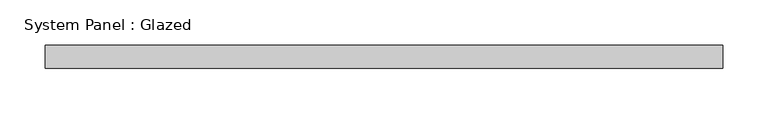
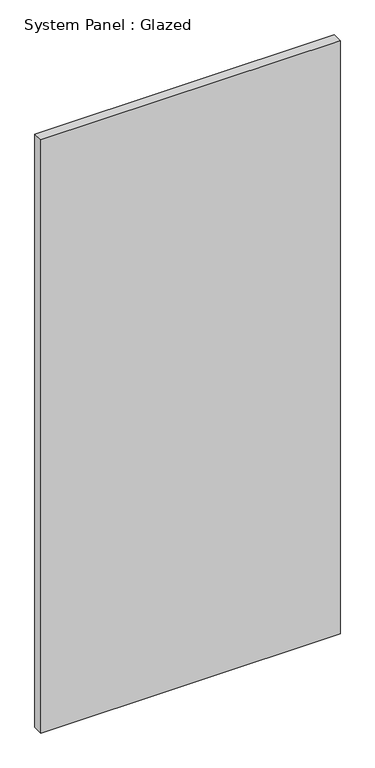
"""IFC4 building model written with IfcOpenShell, lengths in millimetres: plate geometry, System Panel : Glazed."""

from ifc_helpers import new_model, si_unit, origin, origin_with_axes, place, context, project, spatial, polyline, outline, extrude, source, transform, mapped, element, save


def system_panel_glazed_23add07f(model_context):
    return source(origin(), model_context, "Body", "SweptSolid", [
        extrude(outline(polyline([(374.65, 19.05), (-374.65, 19.05), (-374.65, 44.45), (374.65, 44.45), (374.65, 19.05)])), origin_with_axes(), (0.0, 0.0, 1.0), 1570.4525236),
    ])


if __name__ == "__main__":
    model = new_model("IFC4")
    model_context = context("Model", 3, world=origin())
    ifc_project = project(units=[si_unit("LENGTHUNIT", "METRE", prefix="MILLI")], contexts=[model_context])
    site = spatial("IfcSite", under=ifc_project)
    building = spatial("IfcBuilding", under=site)
    placement = place(None, origin())
    system_panel_glazed_shape = system_panel_glazed_23add07f(model_context)
    element("IfcPlate", 1, ObjectType="System Panel : Glazed", at=placement, inside=building, context=model_context, shape_type="MappedRepresentation", body=[
        mapped(system_panel_glazed_shape, transform((0.0, 0.0, 0.0), x_axis=(1.0, 0.0, 0.0), y_axis=(0.0, 1.0, 0.0), z_axis=(0.0, 0.0, 1.0))),
    ])
    save(model, "model.ifc")

# Revit data of these elements
# Type "System Panel : Glazed"
#   Construction Type Id = "GSP4R"
#   Analytic Construction = "1/8 in Pilkington single glazing"
#   Visual Light Transmittance = 0.9
#   Solar Heat Gain Coefficient = 0.86
#   Heat Transfer Coefficient (U) = 1.18115 BTU/(h·ft²·°F)
#   Define Thermal Properties by = 1
# Element 1 (IfcPlate, "System Panel : Glazed")
#   Materials on its faces: "Glass"
# Materials
#   "Glass": class "Glass", colour RGB 0 128 192, transparency 0.75, Description = "Soda Lime Glass", Cost = 0
